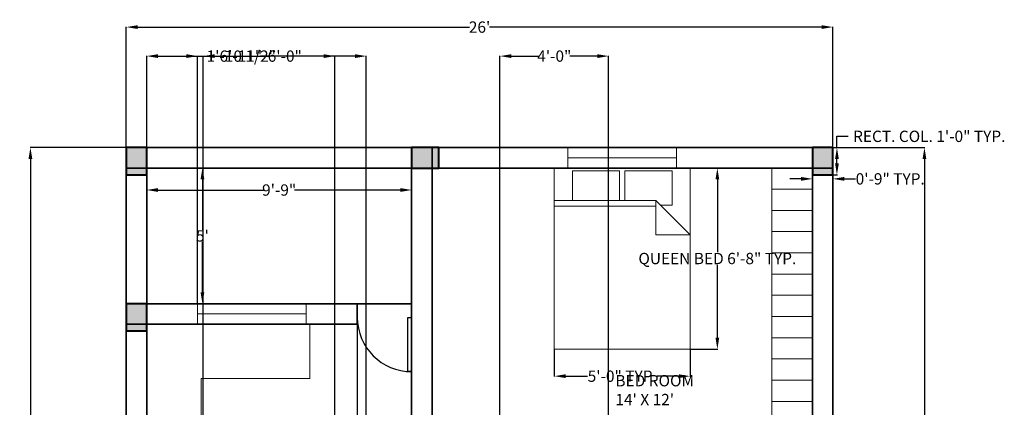
# Model space of a CAD drawing. Units: inches. Extents: x -54 to 881, y -122 to 681.
# Tile 3 of 6: x -47 to 388, y 509 to 681. Entities that reach past the tile are written whole.
import ezdxf

# ---------------------------------------------------------------- set-up
doc = ezdxf.new("R2010")
doc.units = ezdxf.units.IN
doc.header["$MEASUREMENT"] = 0
for name, color, linetype, lineweight in [('A-ANNO-DIMS', 2, 'Continuous', 18), ('A-DOOR', 3, 'Continuous', 25), ('A-FLOR-CASE', 8, 'Continuous', 18), ('A-FURN', 8, 'Continuous', 18), ('A-GLAZ', 4, 'Continuous', 20), ('A-WALL', 7, 'Continuous', 35)]:
    doc.layers.add(name, color=color, linetype=linetype, lineweight=lineweight)
doc.layers.add('A-AREA-IDEN', color=217, linetype='Continuous', lineweight=18, true_color=0x93278f)
doc.layers.add('A-COLS', color=240, linetype='Continuous', lineweight=40, true_color=0xed1f24)
doc.styles.get("Standard").update_dxf_attribs({"font": 'arial.ttf'})
doc.dimstyles.get("Standard").update_dxf_attribs({"dimtxt": 5, "dimasz": 5, "dimexe": 0.18, "dimexo": 0.0625, "dimgap": 0.09, "dimtad": 0, "dimtih": 1, "dimtoh": 1, "dimdec": 0, "dimzin": 0, "dimdsep": 46, "dimlunit": 3, "dimtxsty": 'Standard', "dimcen": 0.09, "dimadec": 0, "dimazin": 0, "dimtfac": 1, "dimtdec": 0, "dimtofl": 0, "dimtmove": 0, "dimatfit": 3, "dimfxl": 1, "dimtolj": 1, "dimtzin": 0, "dimarcsym": 0})

# ---------------------------------------------------------------- blocks, each defined once
blk = doc.blocks.new('*D1')
at = {"layer": 'A-ANNO-DIMS', "color": 0, "lineweight": -2, "transparency": 16777216}
for p, q in [((9, 614.94), (9, 605.09)), ((126, 614.94), (126, 605.09)), ((14, 605.27), (60.76, 605.27)), ((121, 605.27), (74.24, 605.27))]:
    blk.add_line(p, q, dxfattribs=at)
at = {"layer": 'A-ANNO-DIMS', "color": 0, "transparency": 16777216}
for points in [[(14, 606.11), (14, 604.44), (9, 605.27)], [(121, 606.11), (121, 604.44), (126, 605.27)]]:
    blk.add_solid(points, dxfattribs=at)
at = {"layer": 'Defpoints', "color": 0, "transparency": 16777216}
for p in [(9, 615), (126, 615), (126, 605.27)]:
    blk.add_point(p, dxfattribs=at)
at = {"layer": 'A-ANNO-DIMS', "color": 0, "transparency": 16777216, "insert": (67.5, 605.27), "char_height": 5, "attachment_point": 5}
blk.add_mtext('\\A1;9\'-9"', dxfattribs=at)
blk = doc.blocks.new('*D2')
at = {"layer": 'A-ANNO-DIMS', "color": 0, "lineweight": -2, "transparency": 16777216}
for p, q in [((-0.06, 624), (-42.51, 624)), ((-42.33, 619), (-42.33, 374.6)), ((-42.33, 125), (-42.33, 369.4)), ((-0.06, 120), (-42.51, 120))]:
    blk.add_line(p, q, dxfattribs=at)
at = {"layer": 'A-ANNO-DIMS', "color": 0, "transparency": 16777216}
for points in [[(-43.17, 619), (-41.5, 619), (-42.33, 624)], [(-43.17, 125), (-41.5, 125), (-42.33, 120)]]:
    blk.add_solid(points, dxfattribs=at)
at = {"layer": 'Defpoints', "color": 0, "transparency": 16777216}
for p in [(0, 624), (-42.33, 120), (0, 120)]:
    blk.add_point(p, dxfattribs=at)
at = {"layer": 'A-ANNO-DIMS', "color": 0, "transparency": 16777216, "insert": (-42.33, 372), "char_height": 5, "attachment_point": 5}
blk.add_mtext("\\A1;42'", dxfattribs=at)
blk = doc.blocks.new('*D3')
at = {"layer": 'A-ANNO-DIMS', "color": 0, "lineweight": -2, "transparency": 16777216}
for p, q in [((9.06, 615), (33.81, 615)), ((33.63, 610), (33.63, 587.63)), ((33.63, 560), (33.63, 582.37)), ((9.06, 555), (33.81, 555))]:
    blk.add_line(p, q, dxfattribs=at)
at = {"layer": 'A-ANNO-DIMS', "color": 0, "transparency": 16777216}
for points in [[(32.8, 610), (34.46, 610), (33.63, 615)], [(32.8, 560), (34.46, 560), (33.63, 555)]]:
    blk.add_solid(points, dxfattribs=at)
at = {"layer": 'Defpoints', "color": 0, "transparency": 16777216}
for p in [(9, 615), (9, 555), (33.63, 555)]:
    blk.add_point(p, dxfattribs=at)
at = {"layer": 'A-ANNO-DIMS', "color": 0, "transparency": 16777216, "insert": (33.63, 585), "char_height": 5, "attachment_point": 5}
blk.add_mtext("\\A1;5'", dxfattribs=at)
blk = doc.blocks.new('Bed - Queen')
for p, q in [((0, -80.00003), (0, 0)), ((0, 0), (59.99999, 0)), ((59.99999, 0), (59.99999, -80.00003)), ((7.99999, -1.2), (28.79998, -1.2)), ((7.99999, -14.4), (7.99999, -1.2)), ((28.79998, -1.2), (28.79998, -14.4)), ((31.19999, -1.2), (51.99999, -1.2)), ((31.19999, -14.4), (31.19999, -1.2)), ((51.99999, -1.2), (51.99999, -16.4)), ((0, -14.4), (44.8, -14.4)), ((44.8, -16.8), (0, -16.8)), ((59.99999, -29.6), (44.8, -14.4)), ((44.8, -14.4), (44.8, -29.6)), ((51.99999, -16.4), (46.79936, -16.4)), ((44.8, -29.6), (59.99999, -29.6)), ((59.99999, -80.00003), (0, -80.00003))]:
    blk.add_line(p, q)
blk = doc.blocks.new('*U13')
for p, q in [((0, 0), (0, -6)), ((24, 0), (24, -6))]:
    blk.add_line(p, q)
blk.add_lwpolyline([(0, 0), (0, 24), (1.75, 24), (1.75, 0)], close=True)
blk.add_arc((0, 0), 24, 0, 90)
blk = doc.blocks.new('*D21')
at = {"layer": 'A-ANNO-DIMS', "color": 0, "lineweight": -2, "transparency": 16777216}
for p, q in [((0, 624.06), (0, 677.45)), ((5, 677.27), (151.62, 677.27)), ((307, 677.27), (160.38, 677.27)), ((312, 624.06), (312, 677.45))]:
    blk.add_line(p, q, dxfattribs=at)
at = {"layer": 'A-ANNO-DIMS', "color": 0, "transparency": 16777216}
for points in [[(5, 678.11), (5, 676.44), (0, 677.27)], [(307, 678.11), (307, 676.44), (312, 677.27)]]:
    blk.add_solid(points, dxfattribs=at)
at = {"layer": 'Defpoints', "color": 0, "transparency": 16777216}
for p in [(312, 677.27), (0, 624), (312, 624)]:
    blk.add_point(p, dxfattribs=at)
at = {"layer": 'A-ANNO-DIMS', "color": 0, "transparency": 16777216, "insert": (156, 677.27), "char_height": 5, "attachment_point": 5}
blk.add_mtext("\\A1;26'", dxfattribs=at)
blk = doc.blocks.new('WIN-48X9')
for p, q in [((0, 0), (0, 9)), ((48, 0), (48, 9)), ((0, 4.5), (48, 4.5))]:
    blk.add_line(p, q)
blk = doc.blocks.new('KITCHEN-COUNTER-L')
for p, q in [((48, 101), (48, 125)), ((0, 0), (0, 101)), ((0, 101), (48, 101))]:
    blk.add_line(p, q)
blk = doc.blocks.new('STORAGE-RACK-144X18')
for p, q in [((0, 144), (18, 144)), ((0, 0), (0, 144)), ((0, 134.625), (18, 134.625)), ((0, 125.25), (18, 125.25)), ((0, 115.875), (18, 115.875)), ((0, 106.5), (18, 106.5)), ((0, 97.125), (18, 97.125)), ((0, 87.75), (18, 87.75)), ((0, 78.375), (18, 78.375)), ((0, 69), (18, 69)), ((0, 59.625), (18, 59.625)), ((0, 50.25), (18, 50.25)), ((0, 40.875), (18, 40.875)), ((0, 31.5), (18, 31.5)), ((0, 22.125), (18, 22.125)), ((0, 12.75), (18, 12.75)), ((0, 3.375), (18, 3.375))]:
    blk.add_line(p, q)
blk = doc.blocks.new('COL-9X12')
h = blk.add_hatch(color=256)
h.dxf.hatch_style = 1
h.paths.add_polyline_path([(9, 12), (0, 12), (0, 0), (9, 0)])
blk.add_lwpolyline([(0, 0), (9, 0), (9, 12), (0, 12)], close=True)
blk = doc.blocks.new('*D40')
at = {"layer": 'A-ANNO-DIMS', "color": 0, "lineweight": -2, "transparency": 16777216}
for p, q in [((313.8, 624), (313.8, 629)), ((313.8, 629), (318.8, 629)), ((312.06, 624), (313.98, 624)), ((313.8, 617), (313.8, 619)), ((312.06, 612), (313.98, 612))]:
    blk.add_line(p, q, dxfattribs=at)
at = {"layer": 'A-ANNO-DIMS', "color": 0, "transparency": 16777216}
for points in [[(312.97, 619), (314.63, 619), (313.8, 624)], [(312.97, 617), (314.63, 617), (313.8, 612)]]:
    blk.add_solid(points, dxfattribs=at)
at = {"layer": 'Defpoints', "color": 0, "transparency": 16777216}
for p in [(312, 624), (313.8, 624), (312, 612)]:
    blk.add_point(p, dxfattribs=at)
at = {"layer": 'A-ANNO-DIMS', "color": 0, "transparency": 16777216, "insert": (354.57, 629), "char_height": 5, "attachment_point": 5}
blk.add_mtext('\\A1;RECT. COL. 1\'-0" TYP.', dxfattribs=at)
blk = doc.blocks.new('*D41')
at = {"layer": 'A-ANNO-DIMS', "color": 0, "lineweight": -2, "transparency": 16777216}
for p, q in [((298, 610.2), (293, 610.2)), ((303, 611.94), (303, 610.02)), ((312, 611.94), (312, 610.02)), ((317, 610.2), (322, 610.2))]:
    blk.add_line(p, q, dxfattribs=at)
at = {"layer": 'A-ANNO-DIMS', "color": 0, "transparency": 16777216}
for points in [[(298, 611.03), (298, 609.37), (303, 610.2)], [(317, 611.03), (317, 609.37), (312, 610.2)]]:
    blk.add_solid(points, dxfattribs=at)
at = {"layer": 'Defpoints', "color": 0, "transparency": 16777216}
for p in [(303, 612), (312, 612), (312, 610.2)]:
    blk.add_point(p, dxfattribs=at)
at = {"layer": 'A-ANNO-DIMS', "color": 0, "transparency": 16777216, "insert": (337.33, 610.2), "char_height": 5, "attachment_point": 5}
blk.add_mtext('\\A1;0\'-9" TYP.', dxfattribs=at)
blk = doc.blocks.new('*D50')
at = {"layer": 'A-ANNO-DIMS', "color": 0, "lineweight": -2, "transparency": 16777216}
for p, q in [((249.06, 615), (261.18, 615)), ((261, 610), (261, 577.83)), ((261, 540), (261, 572.17)), ((249.06, 535), (261.18, 535))]:
    blk.add_line(p, q, dxfattribs=at)
at = {"layer": 'A-ANNO-DIMS', "color": 0, "transparency": 16777216}
for points in [[(260.17, 610), (261.83, 610), (261, 615)], [(260.17, 540), (261.83, 540), (261, 535)]]:
    blk.add_solid(points, dxfattribs=at)
at = {"layer": 'Defpoints', "color": 0, "transparency": 16777216}
for p in [(249, 615), (261, 615), (249, 535)]:
    blk.add_point(p, dxfattribs=at)
at = {"layer": 'A-ANNO-DIMS', "color": 0, "transparency": 16777216, "insert": (261, 575), "char_height": 5, "attachment_point": 5}
blk.add_mtext('\\A1;QUEEN BED 6\'-8" TYP.', dxfattribs=at)
blk = doc.blocks.new('*D51')
at = {"layer": 'A-ANNO-DIMS', "color": 0, "lineweight": -2, "transparency": 16777216}
for p, q in [((189, 534.94), (189, 522.82)), ((249, 534.94), (249, 522.82)), ((194, 523), (203.67, 523)), ((244, 523), (234.33, 523))]:
    blk.add_line(p, q, dxfattribs=at)
at = {"layer": 'A-ANNO-DIMS', "color": 0, "transparency": 16777216}
for points in [[(194, 523.83), (194, 522.17), (189, 523)], [(244, 523.83), (244, 522.17), (249, 523)]]:
    blk.add_solid(points, dxfattribs=at)
at = {"layer": 'Defpoints', "color": 0, "transparency": 16777216}
for p in [(189, 535), (249, 535), (249, 523)]:
    blk.add_point(p, dxfattribs=at)
at = {"layer": 'A-ANNO-DIMS', "color": 0, "transparency": 16777216, "insert": (219, 523), "char_height": 5, "attachment_point": 5}
blk.add_mtext('\\A1;5\'-0" TYP.', dxfattribs=at)
blk = doc.blocks.new('*D74')
at = {"layer": 'A-ANNO-DIMS', "color": 0, "lineweight": -2, "transparency": 16777216}
for p, q in [((312.06, 624), (352.63, 624)), ((352.45, 619), (352.45, 314.64)), ((352.45, 5), (352.45, 309.36)), ((312.06, 0), (352.63, 0))]:
    blk.add_line(p, q, dxfattribs=at)
at = {"layer": 'A-ANNO-DIMS', "color": 0, "transparency": 16777216}
for points in [[(351.62, 619), (353.28, 619), (352.45, 624)], [(351.62, 5), (353.28, 5), (352.45, 0)]]:
    blk.add_solid(points, dxfattribs=at)
at = {"layer": 'Defpoints', "color": 0, "transparency": 16777216}
for p in [(312, 624), (352.45, 624), (312, 0)]:
    blk.add_point(p, dxfattribs=at)
at = {"layer": 'A-ANNO-DIMS', "color": 0, "transparency": 16777216, "insert": (352.45, 312), "char_height": 5, "attachment_point": 5}
blk.add_mtext('\\A1;52\'-0"', dxfattribs=at)
blk = doc.blocks.new('*D76')
at = {"layer": 'A-ANNO-DIMS', "color": 0, "lineweight": -2, "transparency": 16777216}
for p, q in [((126, 548.94), (126, -40.63)), ((102, 545.94), (102, -40.63)), ((107, -40.45), (107.22, -40.45)), ((121, -40.45), (120.78, -40.45))]:
    blk.add_line(p, q, dxfattribs=at)
at = {"layer": 'A-ANNO-DIMS', "color": 0, "transparency": 16777216}
for points in [[(107, -39.62), (107, -41.28), (102, -40.45)], [(121, -39.62), (121, -41.28), (126, -40.45)]]:
    blk.add_solid(points, dxfattribs=at)
at = {"layer": 'Defpoints', "color": 0, "transparency": 16777216}
for p in [(126, 549), (102, 546), (126, -40.45)]:
    blk.add_point(p, dxfattribs=at)
at = {"layer": 'A-ANNO-DIMS', "color": 0, "transparency": 16777216, "insert": (114, -40.45), "char_height": 5, "attachment_point": 5}
blk.add_mtext('\\A1;2\'-0"', dxfattribs=at)
blk = doc.blocks.new('*D80')
at = {"layer": 'A-ANNO-DIMS', "color": 0, "lineweight": -2, "transparency": 16777216}
for p, q in [((9, 555.06), (9, 664.63)), ((14, 664.45), (26.5, 664.45)), ((31.5, 555.07), (31.5, 664.63)), ((31.5, 664.45), (36.5, 664.45))]:
    blk.add_line(p, q, dxfattribs=at)
at = {"layer": 'A-ANNO-DIMS', "color": 0, "transparency": 16777216}
for points in [[(14, 665.28), (14, 663.62), (9, 664.45)], [(26.5, 665.28), (26.5, 663.62), (31.5, 664.45)]]:
    blk.add_solid(points, dxfattribs=at)
at = {"layer": 'Defpoints', "color": 0, "transparency": 16777216}
for p in [(31.5, 664.45), (9, 555), (31.5, 555.01)]:
    blk.add_point(p, dxfattribs=at)
at = {"layer": 'A-ANNO-DIMS', "color": 0, "transparency": 16777216, "insert": (50.77, 664.45), "char_height": 5, "attachment_point": 5}
blk.add_mtext('\\A1;1\'-10 1/2"', dxfattribs=at)
blk = doc.blocks.new('*D85')
at = {"layer": 'A-ANNO-DIMS', "color": 0, "lineweight": -2, "transparency": 16777216}
for p, q in [((33.99, 120.06), (33.99, 664.63)), ((38.99, 664.45), (63.24, 664.45)), ((100.99, 664.45), (76.73, 664.45)), ((105.99, 120.06), (105.99, 664.63))]:
    blk.add_line(p, q, dxfattribs=at)
at = {"layer": 'A-ANNO-DIMS', "color": 0, "transparency": 16777216}
for points in [[(38.99, 665.28), (38.99, 663.62), (33.99, 664.45)], [(100.99, 665.28), (100.99, 663.62), (105.99, 664.45)]]:
    blk.add_solid(points, dxfattribs=at)
at = {"layer": 'Defpoints', "color": 0, "transparency": 16777216}
for p in [(105.99, 664.45), (33.99, 120), (105.99, 120)]:
    blk.add_point(p, dxfattribs=at)
at = {"layer": 'A-ANNO-DIMS', "color": 0, "transparency": 16777216, "insert": (69.99, 664.45), "char_height": 5, "attachment_point": 5}
blk.add_mtext('\\A1;6\'-0"', dxfattribs=at)
blk = doc.blocks.new('*D89')
at = {"layer": 'A-ANNO-DIMS', "color": 0, "lineweight": -2, "transparency": 16777216}
for p, q in [((165, 120.06), (165, 664.63)), ((170, 664.45), (182.16, 664.45)), ((208, 664.45), (195.84, 664.45)), ((213, 120.06), (213, 664.63))]:
    blk.add_line(p, q, dxfattribs=at)
at = {"layer": 'A-ANNO-DIMS', "color": 0, "transparency": 16777216}
for points in [[(170, 665.28), (170, 663.62), (165, 664.45)], [(208, 665.28), (208, 663.62), (213, 664.45)]]:
    blk.add_solid(points, dxfattribs=at)
at = {"layer": 'Defpoints', "color": 0, "transparency": 16777216}
for p in [(213, 664.45), (165, 120), (213, 120)]:
    blk.add_point(p, dxfattribs=at)
at = {"layer": 'A-ANNO-DIMS', "color": 0, "transparency": 16777216, "insert": (189, 664.45), "char_height": 5, "attachment_point": 5}
blk.add_mtext('\\A1;4\'-0"', dxfattribs=at)
blk = doc.blocks.new('*D90')
at = {"layer": 'A-ANNO-DIMS', "color": 0, "lineweight": -2, "transparency": 16777216}
for p, q in [((9, 243.06), (9, 664.63)), ((14, 664.45), (41.88, 664.45)), ((87.14, 664.45), (59.26, 664.45)), ((92.14, 243.06), (92.14, 664.63))]:
    blk.add_line(p, q, dxfattribs=at)
at = {"layer": 'A-ANNO-DIMS', "color": 0, "transparency": 16777216}
for points in [[(14, 665.28), (14, 663.62), (9, 664.45)], [(87.14, 665.28), (87.14, 663.62), (92.14, 664.45)]]:
    blk.add_solid(points, dxfattribs=at)
at = {"layer": 'Defpoints', "color": 0, "transparency": 16777216}
for p in [(92.14, 664.45), (9, 243), (92.14, 243)]:
    blk.add_point(p, dxfattribs=at)
at = {"layer": 'A-ANNO-DIMS', "color": 0, "transparency": 16777216, "insert": (50.57, 664.45), "char_height": 5, "attachment_point": 5}
blk.add_mtext('\\A1;6\'-11"', dxfattribs=at)

msp = doc.modelspace()

# ---------------------------------------------------------------- linework, layer by layer
at = {"layer": 'A-WALL'}
for p, q in [((0, 0), (0, 624)), ((0, 624), (312, 624)), ((9, 546), (9, 624)), ((126, 462), (126, 624)), ((135, 462), (135, 624)), ((312, 0), (312, 624)), ((0, 615), (135, 615)), ((135, 615), (312, 615)), ((303, 471), (303, 615)), ((0, 555), (126, 555)), ((102, 546), (102, 555)), ((0, 546), (102, 546)), ((9, 421), (9, 546))]:
    msp.add_line(p, q, dxfattribs=at)

# ---------------------------------------------------------------- block references
at = {"layer": 'A-COLS'}
for p in [(0, 612), (303, 612), (0, 543)]:
    msp.add_blockref('COL-9X12', p, dxfattribs=at)
at = {"layer": 'A-COLS', "rotation": 270}
msp.add_blockref('COL-9X12', (126, 624), dxfattribs=at)
at = {"layer": 'A-DOOR', "rotation": 180}
msp.add_blockref('*U13', (126, 549), dxfattribs=at)
at = {"layer": 'A-FLOR-CASE'}
for name, p in [('STORAGE-RACK-144X18', (285, 471)), ('KITCHEN-COUNTER-L', (33, 421))]:
    msp.add_blockref(name, p, dxfattribs=at)
at = {"layer": 'A-FURN'}
msp.add_blockref('Bed - Queen', (189, 615), dxfattribs=at)
at = {"layer": 'A-GLAZ'}
for p in [(195, 615), (31.5, 546.01)]:
    msp.add_blockref('WIN-48X9', p, dxfattribs=at)

# ---------------------------------------------------------------- texts
at = {"layer": 'A-AREA-IDEN', "insert": (215.98, 523.5), "char_height": 5, "attachment_point": 1}
msp.add_mtext_dynamic_manual_height_columns("BED ROOM\\P14' X 12'", width=65.2326, gutter_width=1, heights=[0], dxfattribs=at)

# ---------------------------------------------------------------- dimensions: what is measured, and where the dimension line sits
at = {"layer": 'A-ANNO-DIMS'}
for base, p1, p2, override, picture, middle in [((312, 677.27), (0, 624), (312, 624), {"dimclrd": 0, "dimclre": 0, "dimclrt": 0}, '*D21', (156, 677.27)), ((31.5, 664.45), (9, 555), (31.5, 555.01), {"dimdec": 1, "dimlfac": 1, "dimrnd": 0, "dimzin": 1, "dimdsep": 46, "dimlunit": 4, "dimfrac": 2}, '*D80', (50.77, 664.45)), ((92.14, 664.45), (9, 243), (92.14, 243), {"dimdec": 1, "dimlfac": 1, "dimrnd": 0, "dimzin": 1, "dimdsep": 46, "dimlunit": 4, "dimfrac": 2}, '*D90', (50.57, 664.45)), ((105.99, 664.45), (33.99, 120), (105.99, 120), {"dimdec": 1, "dimlfac": 1, "dimrnd": 0, "dimzin": 1, "dimdsep": 46, "dimlunit": 4, "dimfrac": 2}, '*D85', (69.99, 664.45)), ((213, 664.45), (165, 120), (213, 120), {"dimdec": 1, "dimlfac": 1, "dimrnd": 0, "dimzin": 1, "dimdsep": 46, "dimlunit": 4, "dimfrac": 2}, '*D89', (189, 664.45)), ((126, 605.27), (9, 615), (126, 615), {"dimclrd": 0, "dimclre": 0, "dimclrt": 0}, '*D1', (67.5, 605.27)), ((126, -40.45), (102, 546), (126, 549), {"dimdec": 1, "dimlfac": 1, "dimrnd": 0, "dimzin": 1, "dimdsep": 46, "dimlunit": 4, "dimfrac": 2}, '*D76', (114, -40.45))]:
    dim = msp.add_linear_dim(base=base, p1=p1, p2=p2, dimstyle='Standard', override=override, dxfattribs=at)
    dim.commit()
    dim.dimension.update_dxf_attribs({"geometry": picture, "text_midpoint": middle})
for base, p1, p2, text, picture, middle in [((313.8, 624), (312, 612), (312, 624), 'RECT. COL. <> TYP.', '*D40', (354.57, 629)), ((261, 615), (249, 535), (249, 615), 'QUEEN BED <> TYP.', '*D50', (261, 575))]:
    dim = msp.add_linear_dim(base=base, p1=p1, p2=p2, angle=90, text=text, dimstyle='Standard', override={"dimdec": 1, "dimlfac": 1, "dimrnd": 0, "dimzin": 1, "dimdsep": 46, "dimlunit": 4, "dimfrac": 2}, dxfattribs=at)
    dim.commit()
    dim.dimension.update_dxf_attribs({"geometry": picture, "text_midpoint": middle})
for base, p1, p2, override, picture, middle in [((-42.33, 120), (0, 624), (0, 120), {"dimclrd": 0, "dimclre": 0, "dimclrt": 0}, '*D2', (-42.33, 372)), ((352.45, 624), (312, 0), (312, 624), {"dimdec": 1, "dimlfac": 1, "dimrnd": 0, "dimzin": 1, "dimdsep": 46, "dimlunit": 4, "dimfrac": 2}, '*D74', (352.45, 312)), ((33.63, 555), (9, 615), (9, 555), {"dimclrd": 0, "dimclre": 0, "dimclrt": 0}, '*D3', (33.63, 585))]:
    dim = msp.add_linear_dim(base=base, p1=p1, p2=p2, angle=90, dimstyle='Standard', override=override, dxfattribs=at)
    dim.commit()
    dim.dimension.update_dxf_attribs({"geometry": picture, "text_midpoint": middle})
for base, p1, p2, picture, middle in [((312, 610.2), (303, 612), (312, 612), '*D41', (337.33, 610.2)), ((249, 523), (189, 535), (249, 535), '*D51', (219, 523))]:
    dim = msp.add_linear_dim(base=base, p1=p1, p2=p2, text='<> TYP.', dimstyle='Standard', override={"dimdec": 1, "dimlfac": 1, "dimrnd": 0, "dimzin": 1, "dimdsep": 46, "dimlunit": 4, "dimfrac": 2}, dxfattribs=at)
    dim.commit()
    dim.dimension.update_dxf_attribs({"geometry": picture, "text_midpoint": middle})

doc.saveas('drawing.dxf')
